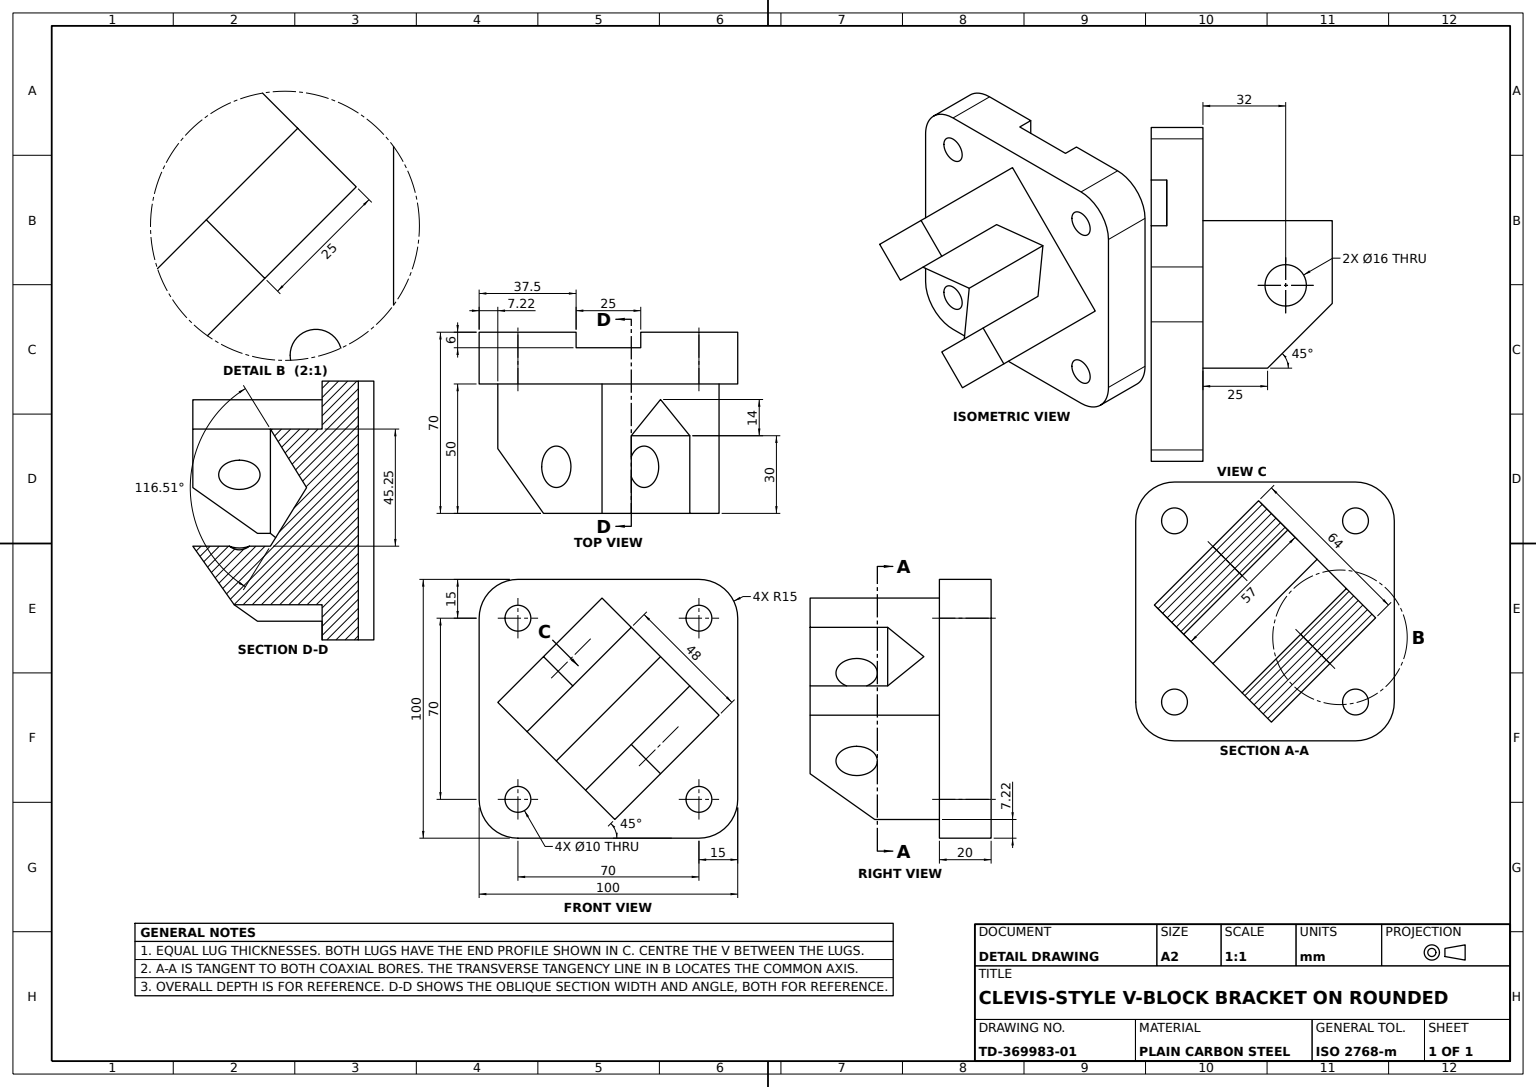
SolidWorks part; units mm, degrees
material "Plain Carbon Steel"
ref_plane "Front Plane" through (0, 0, 0) normal (0, 0, 1) x (1, 0, 0)
ref_plane "Top Plane" through (0, 0, 0) normal (0, 1, 0) x (1, 0, 0)
ref_plane "Right Plane" through (0, 0, 0) normal (1, 0, 0) x (0, 0, -1)
sketch "Base Plate Sketch" plane through (0, 0, 0) normal (0, 0, 1) x (1, 0, 0)
  line L1 (-35, 50) -> (35, 50)
  line L2 (-50, 35) -> (-50, -35)
  line L3 (-35, -50) -> (35, -50)
  line L4 (50, 35) -> (50, -35)
  line L5 (-50, 50) -> (50, -50) construction
  line L6 (-50, -50) -> (50, 50) construction
  arc A0 (-50, -35) -> (-35, -50) centre (-35, -35) ccw
  arc A1 (35, -50) -> (50, -35) centre (35, -35) ccw
  arc A2 (35, 50) -> (50, 35) centre (35, 35) cw
  arc A3 (-35, 50) -> (-50, 35) centre (-35, 35) ccw
  circle A4 centre (-35, 35) radius 5
  circle A5 centre (35, 35) radius 5
  circle A6 centre (35, -35) radius 5
  circle A7 centre (-35, -35) radius 5
  point P0 (0, 0)
  dimension "D3" = 15
  dimension "D4" = 10
  dimension "D1" = 100
  dimension "D2" = 100
extrude "Base Plate" add sketch "Base Plate Sketch" along normal blind 20
sketch "Plate Holes Sketch" plane through (0, -50, 0) normal (0, -1, 0) x (1, 0, 0)
  line L1 (-12.5, -6) -> (12.5, -6)
  line L2 (-12.5, -6) -> (-12.5, 6)
  line L3 (-12.5, 6) -> (12.5, 6)
  line L4 (12.5, -6) -> (12.5, 6)
  line L5 (-12.5, -6) -> (12.5, 6) construction
  line L6 (-12.5, 6) -> (12.5, -6) construction
  point P0 (0, 0)
  dimension "D1" = 12
  dimension "D2" = 25
extrude "Plate Holes Ø12" cut sketch "Plate Holes Sketch" against normal through all both and the other way through all
sketch "Square Boss Sketch" plane through (0, 0, 20) normal (0, 0, 1) x (1, 0, 0)
  line L0 (-42.78, 2.4749) -> (-2.4749, 42.78)
  line L1 (-42.78, 2.4749) -> (2.4749, -42.78)
  line L2 (-2.4749, 42.78) -> (42.78, -2.4749)
  line L3 (2.4749, -42.78) -> (42.78, -2.4749)
  line L4 (-35, -50) -> (35, -50) construction
  line L5 (-45.6066, 45.6066) -> (45.6066, -45.6066) construction
  line L6 (45.6066, 45.6066) -> (-45.6066, -45.6066) construction
  line L7 (50, -35) -> (50, 35) construction
  arc A0 (-35, 50) -> (-50, 35) centre (-35, 35) ccw construction
  arc A1 (35, -50) -> (50, -35) centre (35, -35) ccw construction
  arc A2 (50, 35) -> (35, 50) centre (35, 35) ccw construction
  arc A3 (-50, -35) -> (-35, -50) centre (-35, -35) ccw construction
  dimension "D1" = 45
  dimension "D2" = 57
  dimension "D3" = 28.5
  dimension "D4" = 64
  dimension "D5" = 32
  dimension "D6" = 7.22
  dimension "D7" = 7.22
extrude "Square Boss" add sketch "Square Boss Sketch" along normal blind 50
sketch "Boss Hole Sketch" plane through (22.6274, -22.6274, 0) normal (0.7071, -0.7071, 0) x (0, 0, -1)
  line L0 (-20, -28.5) -> (-20, 28.5) construction
  line L1 (-70, -28.5) -> (-20, -28.5) construction
  circle A0 centre (-52, 3.5) radius 8
  dimension "D1" = 16
  dimension "D2" = 32
  dimension "D3" = 32
extrude "Boss Hole Ø16" cut sketch "Boss Hole Sketch" against normal through all both and the other way through all
chamfer "Boss Chamfer 25x45°" distance 25 angle 45 1 edges at (-20.1525, -20.1525, 70)
sketch "Slot Sketch" plane through (20.1525, 20.1525, 0) normal (0.7071, 0.7071, 0) x (0, 0, -1)
  line L0 (0, 0) -> (-103.125, 0) construction
  line L1 (0, -10.6066) -> (0, 10.6066) construction
  line L2 (-70, 16) -> (-40, 16)
  line L3 (-70, -32) -> (-70, 32) construction
  line L4 (-40, 16) -> (-26, 0)
  line L5 (-40, -16) -> (-26, 0)
  line L6 (-70, -16) -> (-40, -16)
  line L7 (-20, 10.6066) -> (-20, 60.1041) construction
  line L8 (-20, -32) -> (-20, 32) construction
  line L9 (-70, 16) -> (-70, -16)
  dimension "D1" = 20
  dimension "D2" = 6
  dimension "D3" = 32
  dimension "D4" = 16
extrude "Slot Cut" cut sketch "Slot Sketch" against normal through all both and the other way through all
